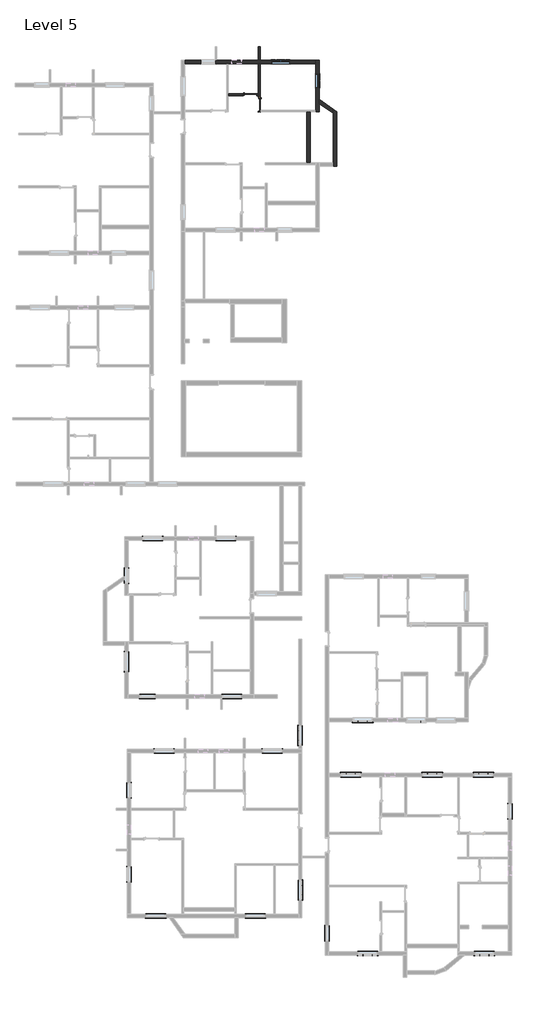
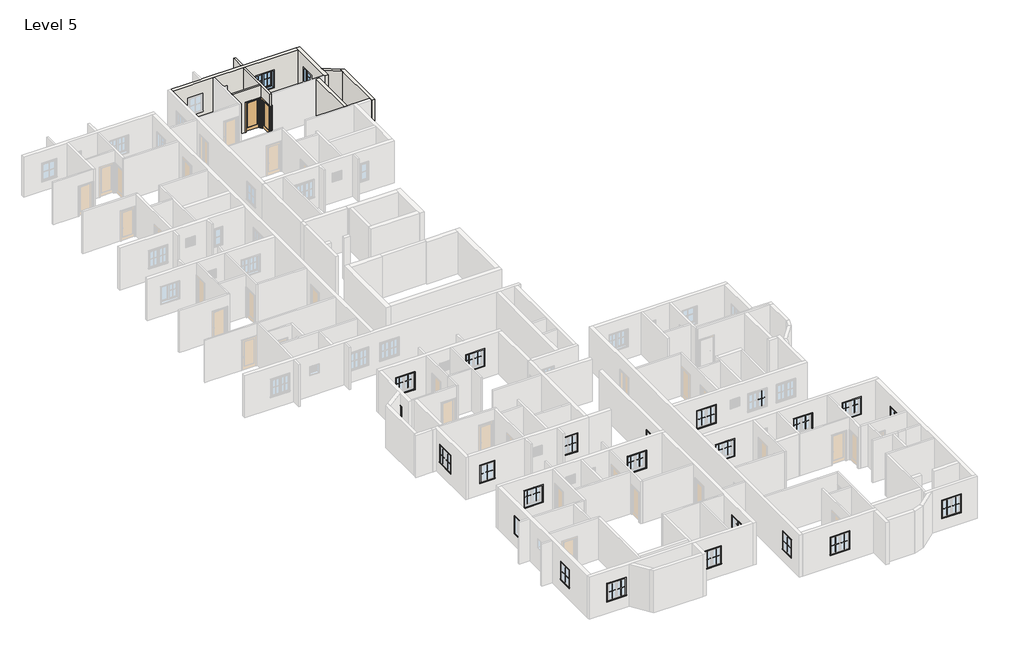
# One storey, part 6 of 7: 82 proxies, 8 walls, 2 doors, 2 windows.
"""IFC4 building model written with IfcOpenShell, lengths in millimetres."""

from ifc_helpers import new_model, si_unit, frame, origin, place, context, project, spatial, polyline, outline, extrude, faceted_brep, transform, mapped, element, save
from components import muntin_pattern_2x2_muntin_pattern_2x2_95b57395, muntin_pattern_2x2_muntin_pattern_2x2_4dfeb3f3, muntin_pattern_2x2_muntin_pattern_2x2_e852a7e4, trim_window_exterior_flat_with_sill_e4b28ec3, trim_window_exterior_flat_with_sill_7cfdd449, trim_window_interior_flat_picture_frame_39ff4276, trim_window_interior_flat_picture_frame_f1e0b15b, door_3c6ab76a, window_272f20d6, window_casement_double_4_x_4_af3140d2

model = new_model("IFC4")

# Units and contexts
model_context = context("Model", 3, world=origin())
ifc_project = project(units=[si_unit("LENGTHUNIT", "METRE", prefix="MILLI")], contexts=[model_context])

# Site, building, storey
site = spatial("IfcSite", under=ifc_project)
building = spatial("IfcBuilding", under=site)
storey = spatial("IfcBuildingStorey", under=building, Name="Level 5", Elevation=6400.8)

# Proxies
placement = place(None, origin())
muntin_pattern_2x2_muntin_pattern_2x2_shape = muntin_pattern_2x2_muntin_pattern_2x2_95b57395(model_context)
element("IfcBuildingElementProxy", 1, Name="Muntin Pattern_2x2 : Muntin Pattern_2x2", ObjectType="Muntin Pattern_2x2 : Muntin Pattern_2x2", at=placement, inside=storey, context=model_context, shape_type="MappedRepresentation", body=[
    mapped(muntin_pattern_2x2_muntin_pattern_2x2_shape, transform((17627.3240531, -20041.5997229, 7385.05), x_axis=(0.0, 1.0, 0.0), y_axis=(-1.0, 0.0, 0.0), z_axis=(0.0, 0.0, 1.0))),
])
element("IfcBuildingElementProxy", 2, Name="Muntin Pattern_2x2 : Muntin Pattern_2x2", ObjectType="Muntin Pattern_2x2 : Muntin Pattern_2x2", at=placement, inside=storey, context=model_context, shape_type="MappedRepresentation", body=[
    mapped(muntin_pattern_2x2_muntin_pattern_2x2_shape, transform((5625.8240531, -28048.9497229, 7385.05), x_axis=(0.0, 1.0, 0.0), y_axis=(-1.0, 0.0, 0.0), z_axis=(0.0, 0.0, 1.0))),
])
element("IfcBuildingElementProxy", 3, Name="Muntin Pattern_2x2 : Muntin Pattern_2x2", ObjectType="Muntin Pattern_2x2 : Muntin Pattern_2x2", at=placement, inside=storey, context=model_context, shape_type="MappedRepresentation", body=[
    mapped(muntin_pattern_2x2_muntin_pattern_2x2_shape, transform((-7378.9759469, -24172.9363256, 7385.05), x_axis=(0.0, 1.0, 0.0), y_axis=(-1.0, 0.0, 0.0), z_axis=(0.0, 0.0, 1.0))),
])
element("IfcBuildingElementProxy", 4, Name="Muntin Pattern_2x2 : Muntin Pattern_2x2", ObjectType="Muntin Pattern_2x2 : Muntin Pattern_2x2", at=placement, inside=storey, context=model_context, shape_type="MappedRepresentation", body=[
    mapped(muntin_pattern_2x2_muntin_pattern_2x2_shape, transform((-7169.4259469, -18656.0038828, 7385.05), x_axis=(0.0, -1.0, 0.0), y_axis=(1.0, 0.0, 0.0), z_axis=(0.0, 0.0, 1.0))),
])
element("IfcBuildingElementProxy", 5, Name="Muntin Pattern_2x2 : Muntin Pattern_2x2", ObjectType="Muntin Pattern_2x2 : Muntin Pattern_2x2", at=placement, inside=storey, context=model_context, shape_type="MappedRepresentation", body=[
    mapped(muntin_pattern_2x2_muntin_pattern_2x2_shape, transform((-6067.7009469, -12594.9288828, 7385.05), x_axis=(-1.0, 0.0, 0.0), y_axis=(0.0, -1.0, 0.0), z_axis=(0.0, 0.0, 1.0))),
])
element("IfcBuildingElementProxy", 6, Name="Muntin Pattern_2x2 : Muntin Pattern_2x2", ObjectType="Muntin Pattern_2x2 : Muntin Pattern_2x2", at=placement, inside=storey, context=model_context, shape_type="MappedRepresentation", body=[
    mapped(muntin_pattern_2x2_muntin_pattern_2x2_shape, transform((-7334.5259469, -4559.0038828, 7385.05), x_axis=(0.0, -1.0, 0.0), y_axis=(1.0, 0.0, 0.0), z_axis=(0.0, 0.0, 1.0))),
])
muntin_pattern_2x2_muntin_pattern_2x2_2_shape = muntin_pattern_2x2_muntin_pattern_2x2_4dfeb3f3(model_context)
element("IfcBuildingElementProxy", 7, Name="Muntin Pattern_2x2 : Muntin Pattern_2x2", ObjectType="Muntin Pattern_2x2 : Muntin Pattern_2x2", at=placement, inside=storey, context=model_context, shape_type="MappedRepresentation", body=[
    mapped(muntin_pattern_2x2_muntin_pattern_2x2_2_shape, transform((11869.4615531, -14158.3247229, 7385.05), x_axis=(-1.0, 0.0, 0.0), y_axis=(0.0, -1.0, 0.0), z_axis=(0.0, 0.0, 1.0))),
])
element("IfcBuildingElementProxy", 8, Name="Muntin Pattern_2x2 : Muntin Pattern_2x2", ObjectType="Muntin Pattern_2x2 : Muntin Pattern_2x2", at=placement, inside=storey, context=model_context, shape_type="MappedRepresentation", body=[
    mapped(muntin_pattern_2x2_muntin_pattern_2x2_2_shape, transform((8364.2615531, -14158.3247229, 7385.05), x_axis=(-1.0, 0.0, 0.0), y_axis=(0.0, -1.0, 0.0), z_axis=(0.0, 0.0, 1.0))),
])
element("IfcBuildingElementProxy", 9, Name="Muntin Pattern_2x2 : Muntin Pattern_2x2", ObjectType="Muntin Pattern_2x2 : Muntin Pattern_2x2", at=placement, inside=storey, context=model_context, shape_type="MappedRepresentation", body=[
    mapped(muntin_pattern_2x2_muntin_pattern_2x2_2_shape, transform((6976.7865531, -17530.1747229, 7385.05), x_axis=(1.0, 0.0, 0.0), y_axis=(0.0, 1.0, 0.0), z_axis=(0.0, 0.0, 1.0))),
])
element("IfcBuildingElementProxy", 10, Name="Muntin Pattern_2x2 : Muntin Pattern_2x2", ObjectType="Muntin Pattern_2x2 : Muntin Pattern_2x2", at=placement, inside=storey, context=model_context, shape_type="MappedRepresentation", body=[
    mapped(muntin_pattern_2x2_muntin_pattern_2x2_2_shape, transform((12323.4865531, -17530.1747229, 7385.05), x_axis=(1.0, 0.0, 0.0), y_axis=(0.0, 1.0, 0.0), z_axis=(0.0, 0.0, 1.0))),
])
element("IfcBuildingElementProxy", 11, Name="Muntin Pattern_2x2 : Muntin Pattern_2x2", ObjectType="Muntin Pattern_2x2 : Muntin Pattern_2x2", at=placement, inside=storey, context=model_context, shape_type="MappedRepresentation", body=[
    mapped(muntin_pattern_2x2_muntin_pattern_2x2_2_shape, transform((15682.6365531, -17530.1747229, 7385.05), x_axis=(1.0, 0.0, 0.0), y_axis=(0.0, 1.0, 0.0), z_axis=(0.0, 0.0, 1.0))),
])
element("IfcBuildingElementProxy", 12, Name="Muntin Pattern_2x2 : Muntin Pattern_2x2", ObjectType="Muntin Pattern_2x2 : Muntin Pattern_2x2", at=placement, inside=storey, context=model_context, shape_type="MappedRepresentation", body=[
    mapped(muntin_pattern_2x2_muntin_pattern_2x2_2_shape, transform((16349.3865531, -29474.5247229, 7385.05), x_axis=(-1.0, 0.0, 0.0), y_axis=(0.0, -1.0, 0.0), z_axis=(0.0, 0.0, 1.0))),
])
element("IfcBuildingElementProxy", 13, Name="Muntin Pattern_2x2 : Muntin Pattern_2x2", ObjectType="Muntin Pattern_2x2 : Muntin Pattern_2x2", at=placement, inside=storey, context=model_context, shape_type="MappedRepresentation", body=[
    mapped(muntin_pattern_2x2_muntin_pattern_2x2_2_shape, transform((8694.4615531, -29474.5247229, 7385.05), x_axis=(-1.0, 0.0, 0.0), y_axis=(0.0, -1.0, 0.0), z_axis=(0.0, 0.0, 1.0))),
])
element("IfcBuildingElementProxy", 14, Name="Muntin Pattern_2x2 : Muntin Pattern_2x2", ObjectType="Muntin Pattern_2x2 : Muntin Pattern_2x2", at=placement, inside=storey, context=model_context, shape_type="MappedRepresentation", body=[
    mapped(muntin_pattern_2x2_muntin_pattern_2x2_2_shape, transform((4070.0740531, -24902.8163828, 7385.05), x_axis=(0.0, -1.0, 0.0), y_axis=(1.0, 0.0, 0.0), z_axis=(0.0, 0.0, 1.0))),
])
element("IfcBuildingElementProxy", 15, Name="Muntin Pattern_2x2 : Muntin Pattern_2x2", ObjectType="Muntin Pattern_2x2 : Muntin Pattern_2x2", at=placement, inside=storey, context=model_context, shape_type="MappedRepresentation", body=[
    mapped(muntin_pattern_2x2_muntin_pattern_2x2_2_shape, transform((1325.2865531, -26996.7288828, 7385.05), x_axis=(-1.0, 0.0, 0.0), y_axis=(0.0, -1.0, 0.0), z_axis=(0.0, 0.0, 1.0))),
])
element("IfcBuildingElementProxy", 16, Name="Muntin Pattern_2x2 : Muntin Pattern_2x2", ObjectType="Muntin Pattern_2x2 : Muntin Pattern_2x2", at=placement, inside=storey, context=model_context, shape_type="MappedRepresentation", body=[
    mapped(muntin_pattern_2x2_muntin_pattern_2x2_2_shape, transform((-5208.8634469, -26996.7288828, 7385.05), x_axis=(-1.0, 0.0, 0.0), y_axis=(0.0, -1.0, 0.0), z_axis=(0.0, 0.0, 1.0))),
])
element("IfcBuildingElementProxy", 17, Name="Muntin Pattern_2x2 : Muntin Pattern_2x2", ObjectType="Muntin Pattern_2x2 : Muntin Pattern_2x2", at=placement, inside=storey, context=model_context, shape_type="MappedRepresentation", body=[
    mapped(muntin_pattern_2x2_muntin_pattern_2x2_2_shape, transform((1823.7615531, -15966.7788828, 7385.05), x_axis=(1.0, 0.0, 0.0), y_axis=(0.0, 1.0, 0.0), z_axis=(0.0, 0.0, 1.0))),
])
element("IfcBuildingElementProxy", 18, Name="Muntin Pattern_2x2 : Muntin Pattern_2x2", ObjectType="Muntin Pattern_2x2 : Muntin Pattern_2x2", at=placement, inside=storey, context=model_context, shape_type="MappedRepresentation", body=[
    mapped(muntin_pattern_2x2_muntin_pattern_2x2_2_shape, transform((-5272.3634469, -15966.7788828, 7385.05), x_axis=(1.0, 0.0, 0.0), y_axis=(0.0, 1.0, 0.0), z_axis=(0.0, 0.0, 1.0))),
])
element("IfcBuildingElementProxy", 19, Name="Muntin Pattern_2x2 : Muntin Pattern_2x2", ObjectType="Muntin Pattern_2x2 : Muntin Pattern_2x2", at=placement, inside=storey, context=model_context, shape_type="MappedRepresentation", body=[
    mapped(muntin_pattern_2x2_muntin_pattern_2x2_2_shape, transform((3860.5240531, -15358.7663828, 7385.05), x_axis=(0.0, 1.0, 0.0), y_axis=(-1.0, 0.0, 0.0), z_axis=(0.0, 0.0, 1.0))),
])
element("IfcBuildingElementProxy", 20, Name="Muntin Pattern_2x2 : Muntin Pattern_2x2", ObjectType="Muntin Pattern_2x2 : Muntin Pattern_2x2", at=placement, inside=storey, context=model_context, shape_type="MappedRepresentation", body=[
    mapped(muntin_pattern_2x2_muntin_pattern_2x2_2_shape, transform((-239.9884469, -12594.9288828, 7385.05), x_axis=(-1.0, 0.0, 0.0), y_axis=(0.0, -1.0, 0.0), z_axis=(0.0, 0.0, 1.0))),
])
element("IfcBuildingElementProxy", 21, Name="Muntin Pattern_2x2 : Muntin Pattern_2x2", ObjectType="Muntin Pattern_2x2 : Muntin Pattern_2x2", at=placement, inside=storey, context=model_context, shape_type="MappedRepresentation", body=[
    mapped(muntin_pattern_2x2_muntin_pattern_2x2_2_shape, transform((-7544.0759469, -10513.7163828, 7385.05), x_axis=(0.0, 1.0, 0.0), y_axis=(-1.0, 0.0, 0.0), z_axis=(0.0, 0.0, 1.0))),
])
element("IfcBuildingElementProxy", 22, Name="Muntin Pattern_2x2 : Muntin Pattern_2x2", ObjectType="Muntin Pattern_2x2 : Muntin Pattern_2x2", at=placement, inside=storey, context=model_context, shape_type="MappedRepresentation", body=[
    mapped(muntin_pattern_2x2_muntin_pattern_2x2_2_shape, transform((-6021.6634469, -2022.1788828, 7385.05), x_axis=(1.0, 0.0, 0.0), y_axis=(0.0, 1.0, 0.0), z_axis=(0.0, 0.0, 1.0))),
])
element("IfcBuildingElementProxy", 23, Name="Muntin Pattern_2x2 : Muntin Pattern_2x2", ObjectType="Muntin Pattern_2x2 : Muntin Pattern_2x2", at=placement, inside=storey, context=model_context, shape_type="MappedRepresentation", body=[
    mapped(muntin_pattern_2x2_muntin_pattern_2x2_2_shape, transform((-1221.0634469, -2022.1788828, 7385.05), x_axis=(1.0, 0.0, 0.0), y_axis=(0.0, 1.0, 0.0), z_axis=(0.0, 0.0, 1.0))),
])
muntin_pattern_2x2_muntin_pattern_2x2_3_shape = muntin_pattern_2x2_muntin_pattern_2x2_e852a7e4(model_context)
element("IfcBuildingElementProxy", 24, Name="Muntin Pattern_2x2 : Muntin Pattern_2x2", ObjectType="Muntin Pattern_2x2 : Muntin Pattern_2x2", at=placement, inside=storey, context=model_context, shape_type="MappedRepresentation", body=[
    mapped(muntin_pattern_2x2_muntin_pattern_2x2_3_shape, transform((7757.8365531, -14158.3247229, 7385.05), x_axis=(1.0, 0.0, 0.0), y_axis=(0.0, 1.0, 0.0), z_axis=(0.0, 0.0, 1.0))),
])
element("IfcBuildingElementProxy", 25, Name="Muntin Pattern_2x2 : Muntin Pattern_2x2", ObjectType="Muntin Pattern_2x2 : Muntin Pattern_2x2", at=placement, inside=storey, context=model_context, shape_type="MappedRepresentation", body=[
    mapped(muntin_pattern_2x2_muntin_pattern_2x2_3_shape, transform((7583.2115531, -17530.1747229, 7385.05), x_axis=(-1.0, 0.0, 0.0), y_axis=(0.0, -1.0, 0.0), z_axis=(0.0, 0.0, 1.0))),
])
element("IfcBuildingElementProxy", 26, Name="Muntin Pattern_2x2 : Muntin Pattern_2x2", ObjectType="Muntin Pattern_2x2 : Muntin Pattern_2x2", at=placement, inside=storey, context=model_context, shape_type="MappedRepresentation", body=[
    mapped(muntin_pattern_2x2_muntin_pattern_2x2_3_shape, transform((12929.9115531, -17530.1747229, 7385.05), x_axis=(-1.0, 0.0, 0.0), y_axis=(0.0, -1.0, 0.0), z_axis=(0.0, 0.0, 1.0))),
])
element("IfcBuildingElementProxy", 27, Name="Muntin Pattern_2x2 : Muntin Pattern_2x2", ObjectType="Muntin Pattern_2x2 : Muntin Pattern_2x2", at=placement, inside=storey, context=model_context, shape_type="MappedRepresentation", body=[
    mapped(muntin_pattern_2x2_muntin_pattern_2x2_3_shape, transform((16289.0615531, -17530.1747229, 7385.05), x_axis=(-1.0, 0.0, 0.0), y_axis=(0.0, -1.0, 0.0), z_axis=(0.0, 0.0, 1.0))),
])
element("IfcBuildingElementProxy", 28, Name="Muntin Pattern_2x2 : Muntin Pattern_2x2", ObjectType="Muntin Pattern_2x2 : Muntin Pattern_2x2", at=placement, inside=storey, context=model_context, shape_type="MappedRepresentation", body=[
    mapped(muntin_pattern_2x2_muntin_pattern_2x2_3_shape, transform((15742.9615531, -29474.5247229, 7385.05), x_axis=(1.0, 0.0, 0.0), y_axis=(0.0, 1.0, 0.0), z_axis=(0.0, 0.0, 1.0))),
])
element("IfcBuildingElementProxy", 29, Name="Muntin Pattern_2x2 : Muntin Pattern_2x2", ObjectType="Muntin Pattern_2x2 : Muntin Pattern_2x2", at=placement, inside=storey, context=model_context, shape_type="MappedRepresentation", body=[
    mapped(muntin_pattern_2x2_muntin_pattern_2x2_3_shape, transform((8088.0365531, -29474.5247229, 7385.05), x_axis=(1.0, 0.0, 0.0), y_axis=(0.0, 1.0, 0.0), z_axis=(0.0, 0.0, 1.0))),
])
element("IfcBuildingElementProxy", 30, Name="Muntin Pattern_2x2 : Muntin Pattern_2x2", ObjectType="Muntin Pattern_2x2 : Muntin Pattern_2x2", at=placement, inside=storey, context=model_context, shape_type="MappedRepresentation", body=[
    mapped(muntin_pattern_2x2_muntin_pattern_2x2_3_shape, transform((4070.0740531, -25509.2413828, 7385.05), x_axis=(0.0, 1.0, 0.0), y_axis=(-1.0, 0.0, 0.0), z_axis=(0.0, 0.0, 1.0))),
])
element("IfcBuildingElementProxy", 31, Name="Muntin Pattern_2x2 : Muntin Pattern_2x2", ObjectType="Muntin Pattern_2x2 : Muntin Pattern_2x2", at=placement, inside=storey, context=model_context, shape_type="MappedRepresentation", body=[
    mapped(muntin_pattern_2x2_muntin_pattern_2x2_3_shape, transform((718.8615531, -26996.7288828, 7385.05), x_axis=(1.0, 0.0, 0.0), y_axis=(0.0, 1.0, 0.0), z_axis=(0.0, 0.0, 1.0))),
])
element("IfcBuildingElementProxy", 32, Name="Muntin Pattern_2x2 : Muntin Pattern_2x2", ObjectType="Muntin Pattern_2x2 : Muntin Pattern_2x2", at=placement, inside=storey, context=model_context, shape_type="MappedRepresentation", body=[
    mapped(muntin_pattern_2x2_muntin_pattern_2x2_3_shape, transform((-5815.2884469, -26996.7288828, 7385.05), x_axis=(1.0, 0.0, 0.0), y_axis=(0.0, 1.0, 0.0), z_axis=(0.0, 0.0, 1.0))),
])
element("IfcBuildingElementProxy", 33, Name="Muntin Pattern_2x2 : Muntin Pattern_2x2", ObjectType="Muntin Pattern_2x2 : Muntin Pattern_2x2", at=placement, inside=storey, context=model_context, shape_type="MappedRepresentation", body=[
    mapped(muntin_pattern_2x2_muntin_pattern_2x2_3_shape, transform((2430.1865531, -15966.7788828, 7385.05), x_axis=(-1.0, 0.0, 0.0), y_axis=(0.0, -1.0, 0.0), z_axis=(0.0, 0.0, 1.0))),
])
element("IfcBuildingElementProxy", 34, Name="Muntin Pattern_2x2 : Muntin Pattern_2x2", ObjectType="Muntin Pattern_2x2 : Muntin Pattern_2x2", at=placement, inside=storey, context=model_context, shape_type="MappedRepresentation", body=[
    mapped(muntin_pattern_2x2_muntin_pattern_2x2_3_shape, transform((-4665.9384469, -15966.7788828, 7385.05), x_axis=(-1.0, 0.0, 0.0), y_axis=(0.0, -1.0, 0.0), z_axis=(0.0, 0.0, 1.0))),
])
element("IfcBuildingElementProxy", 35, Name="Muntin Pattern_2x2 : Muntin Pattern_2x2", ObjectType="Muntin Pattern_2x2 : Muntin Pattern_2x2", at=placement, inside=storey, context=model_context, shape_type="MappedRepresentation", body=[
    mapped(muntin_pattern_2x2_muntin_pattern_2x2_3_shape, transform((3860.5240531, -14752.3413828, 7385.05), x_axis=(0.0, -1.0, 0.0), y_axis=(1.0, 0.0, 0.0), z_axis=(0.0, 0.0, 1.0))),
])
element("IfcBuildingElementProxy", 36, Name="Muntin Pattern_2x2 : Muntin Pattern_2x2", ObjectType="Muntin Pattern_2x2 : Muntin Pattern_2x2", at=placement, inside=storey, context=model_context, shape_type="MappedRepresentation", body=[
    mapped(muntin_pattern_2x2_muntin_pattern_2x2_3_shape, transform((-846.4134469, -12594.9288828, 7385.05), x_axis=(1.0, 0.0, 0.0), y_axis=(0.0, 1.0, 0.0), z_axis=(0.0, 0.0, 1.0))),
])
element("IfcBuildingElementProxy", 37, Name="Muntin Pattern_2x2 : Muntin Pattern_2x2", ObjectType="Muntin Pattern_2x2 : Muntin Pattern_2x2", at=placement, inside=storey, context=model_context, shape_type="MappedRepresentation", body=[
    mapped(muntin_pattern_2x2_muntin_pattern_2x2_3_shape, transform((-7544.0759469, -9907.2913828, 7385.05), x_axis=(0.0, -1.0, 0.0), y_axis=(1.0, 0.0, 0.0), z_axis=(0.0, 0.0, 1.0))),
])
element("IfcBuildingElementProxy", 38, Name="Muntin Pattern_2x2 : Muntin Pattern_2x2", ObjectType="Muntin Pattern_2x2 : Muntin Pattern_2x2", at=placement, inside=storey, context=model_context, shape_type="MappedRepresentation", body=[
    mapped(muntin_pattern_2x2_muntin_pattern_2x2_3_shape, transform((-5415.2384469, -2022.1788828, 7385.05), x_axis=(-1.0, 0.0, 0.0), y_axis=(0.0, -1.0, 0.0), z_axis=(0.0, 0.0, 1.0))),
])
element("IfcBuildingElementProxy", 39, Name="Muntin Pattern_2x2 : Muntin Pattern_2x2", ObjectType="Muntin Pattern_2x2 : Muntin Pattern_2x2", at=placement, inside=storey, context=model_context, shape_type="MappedRepresentation", body=[
    mapped(muntin_pattern_2x2_muntin_pattern_2x2_3_shape, transform((-614.6384469, -2022.1788828, 7385.05), x_axis=(-1.0, 0.0, 0.0), y_axis=(0.0, -1.0, 0.0), z_axis=(0.0, 0.0, 1.0))),
])
trim_window_exterior_flat_with_sill_shape = trim_window_exterior_flat_with_sill_e4b28ec3(model_context)
element("IfcBuildingElementProxy", 40, Name="Trim-Window-Exterior-Flat : with Sill", ObjectType="Trim-Window-Exterior-Flat : with Sill", at=placement, inside=storey, context=model_context, shape_type="MappedRepresentation", body=[
    mapped(trim_window_exterior_flat_with_sill_shape, transform((17617.7990531, -20041.5997229, 8534.4), x_axis=(0.0, -1.0, 0.0), y_axis=(0.0, 0.0, 1.0), z_axis=(-1.0, 0.0, 0.0))),
])
element("IfcBuildingElementProxy", 41, Name="Trim-Window-Exterior-Flat : with Sill", ObjectType="Trim-Window-Exterior-Flat : with Sill", at=placement, inside=storey, context=model_context, shape_type="MappedRepresentation", body=[
    mapped(trim_window_exterior_flat_with_sill_shape, transform((5616.2990531, -28048.9497229, 8534.4), x_axis=(0.0, -1.0, 0.0), y_axis=(0.0, 0.0, 1.0), z_axis=(-1.0, 0.0, 0.0))),
])
element("IfcBuildingElementProxy", 42, Name="Trim-Window-Exterior-Flat : with Sill", ObjectType="Trim-Window-Exterior-Flat : with Sill", at=placement, inside=storey, context=model_context, shape_type="MappedRepresentation", body=[
    mapped(trim_window_exterior_flat_with_sill_shape, transform((-7388.5009469, -24172.9363256, 8534.4), x_axis=(0.0, -1.0, 0.0), y_axis=(0.0, 0.0, 1.0), z_axis=(-1.0, 0.0, 0.0))),
])
element("IfcBuildingElementProxy", 43, Name="Trim-Window-Exterior-Flat : with Sill", ObjectType="Trim-Window-Exterior-Flat : with Sill", at=placement, inside=storey, context=model_context, shape_type="MappedRepresentation", body=[
    mapped(trim_window_exterior_flat_with_sill_shape, transform((-7159.9009469, -18656.0038828, 8534.4), x_axis=(0.0, 1.0, 0.0), y_axis=(0.0, 0.0, 1.0), z_axis=(1.0, 0.0, 0.0))),
])
element("IfcBuildingElementProxy", 44, Name="Trim-Window-Exterior-Flat : with Sill", ObjectType="Trim-Window-Exterior-Flat : with Sill", at=placement, inside=storey, context=model_context, shape_type="MappedRepresentation", body=[
    mapped(trim_window_exterior_flat_with_sill_shape, transform((-6067.7009469, -12604.4538828, 8534.4), x_axis=(1.0, 0.0, 0.0), y_axis=(0.0, 0.0, 1.0), z_axis=(0.0, -1.0, 0.0))),
])
element("IfcBuildingElementProxy", 45, Name="Trim-Window-Exterior-Flat : with Sill", ObjectType="Trim-Window-Exterior-Flat : with Sill", at=placement, inside=storey, context=model_context, shape_type="MappedRepresentation", body=[
    mapped(trim_window_exterior_flat_with_sill_shape, transform((-7325.0009469, -4559.0038828, 8534.4), x_axis=(0.0, 1.0, 0.0), y_axis=(0.0, 0.0, 1.0), z_axis=(1.0, 0.0, 0.0))),
])
trim_window_exterior_flat_with_sill_2_shape = trim_window_exterior_flat_with_sill_7cfdd449(model_context)
element("IfcBuildingElementProxy", 46, Name="Trim-Window-Exterior-Flat : with Sill", ObjectType="Trim-Window-Exterior-Flat : with Sill", at=placement, inside=storey, context=model_context, shape_type="MappedRepresentation", body=[
    mapped(trim_window_exterior_flat_with_sill_2_shape, transform((8061.0490531, -14167.8497229, 8534.4), x_axis=(1.0, 0.0, 0.0), y_axis=(0.0, 0.0, 1.0), z_axis=(0.0, -1.0, 0.0))),
])
element("IfcBuildingElementProxy", 47, Name="Trim-Window-Exterior-Flat : with Sill", ObjectType="Trim-Window-Exterior-Flat : with Sill", at=placement, inside=storey, context=model_context, shape_type="MappedRepresentation", body=[
    mapped(trim_window_exterior_flat_with_sill_2_shape, transform((7279.9990531, -17520.6497229, 8534.4), x_axis=(-1.0, 0.0, 0.0), y_axis=(0.0, 0.0, 1.0), z_axis=(0.0, 1.0, 0.0))),
])
element("IfcBuildingElementProxy", 48, Name="Trim-Window-Exterior-Flat : with Sill", ObjectType="Trim-Window-Exterior-Flat : with Sill", at=placement, inside=storey, context=model_context, shape_type="MappedRepresentation", body=[
    mapped(trim_window_exterior_flat_with_sill_2_shape, transform((12626.6990531, -17520.6497229, 8534.4), x_axis=(-1.0, 0.0, 0.0), y_axis=(0.0, 0.0, 1.0), z_axis=(0.0, 1.0, 0.0))),
])
element("IfcBuildingElementProxy", 49, Name="Trim-Window-Exterior-Flat : with Sill", ObjectType="Trim-Window-Exterior-Flat : with Sill", at=placement, inside=storey, context=model_context, shape_type="MappedRepresentation", body=[
    mapped(trim_window_exterior_flat_with_sill_2_shape, transform((15985.8490531, -17520.6497229, 8534.4), x_axis=(-1.0, 0.0, 0.0), y_axis=(0.0, 0.0, 1.0), z_axis=(0.0, 1.0, 0.0))),
])
element("IfcBuildingElementProxy", 50, Name="Trim-Window-Exterior-Flat : with Sill", ObjectType="Trim-Window-Exterior-Flat : with Sill", at=placement, inside=storey, context=model_context, shape_type="MappedRepresentation", body=[
    mapped(trim_window_exterior_flat_with_sill_2_shape, transform((16046.1740531, -29484.0497229, 8534.4), x_axis=(1.0, 0.0, 0.0), y_axis=(0.0, 0.0, 1.0), z_axis=(0.0, -1.0, 0.0))),
])
element("IfcBuildingElementProxy", 51, Name="Trim-Window-Exterior-Flat : with Sill", ObjectType="Trim-Window-Exterior-Flat : with Sill", at=placement, inside=storey, context=model_context, shape_type="MappedRepresentation", body=[
    mapped(trim_window_exterior_flat_with_sill_2_shape, transform((8391.2490531, -29484.0497229, 8534.4), x_axis=(1.0, 0.0, 0.0), y_axis=(0.0, 0.0, 1.0), z_axis=(0.0, -1.0, 0.0))),
])
element("IfcBuildingElementProxy", 52, Name="Trim-Window-Exterior-Flat : with Sill", ObjectType="Trim-Window-Exterior-Flat : with Sill", at=placement, inside=storey, context=model_context, shape_type="MappedRepresentation", body=[
    mapped(trim_window_exterior_flat_with_sill_2_shape, transform((4079.5990531, -25206.0288828, 8534.4), x_axis=(0.0, 1.0, 0.0), y_axis=(0.0, 0.0, 1.0), z_axis=(1.0, 0.0, 0.0))),
])
element("IfcBuildingElementProxy", 53, Name="Trim-Window-Exterior-Flat : with Sill", ObjectType="Trim-Window-Exterior-Flat : with Sill", at=placement, inside=storey, context=model_context, shape_type="MappedRepresentation", body=[
    mapped(trim_window_exterior_flat_with_sill_2_shape, transform((1022.0740531, -27006.2538828, 8534.4), x_axis=(1.0, 0.0, 0.0), y_axis=(0.0, 0.0, 1.0), z_axis=(0.0, -1.0, 0.0))),
])
element("IfcBuildingElementProxy", 54, Name="Trim-Window-Exterior-Flat : with Sill", ObjectType="Trim-Window-Exterior-Flat : with Sill", at=placement, inside=storey, context=model_context, shape_type="MappedRepresentation", body=[
    mapped(trim_window_exterior_flat_with_sill_2_shape, transform((-5512.0759469, -27006.2538828, 8534.4), x_axis=(1.0, 0.0, 0.0), y_axis=(0.0, 0.0, 1.0), z_axis=(0.0, -1.0, 0.0))),
])
element("IfcBuildingElementProxy", 55, Name="Trim-Window-Exterior-Flat : with Sill", ObjectType="Trim-Window-Exterior-Flat : with Sill", at=placement, inside=storey, context=model_context, shape_type="MappedRepresentation", body=[
    mapped(trim_window_exterior_flat_with_sill_2_shape, transform((2126.9740531, -15957.2538828, 8534.4), x_axis=(-1.0, 0.0, 0.0), y_axis=(0.0, 0.0, 1.0), z_axis=(0.0, 1.0, 0.0))),
])
element("IfcBuildingElementProxy", 56, Name="Trim-Window-Exterior-Flat : with Sill", ObjectType="Trim-Window-Exterior-Flat : with Sill", at=placement, inside=storey, context=model_context, shape_type="MappedRepresentation", body=[
    mapped(trim_window_exterior_flat_with_sill_2_shape, transform((-4969.1509469, -15957.2538828, 8534.4), x_axis=(-1.0, 0.0, 0.0), y_axis=(0.0, 0.0, 1.0), z_axis=(0.0, 1.0, 0.0))),
])
element("IfcBuildingElementProxy", 57, Name="Trim-Window-Exterior-Flat : with Sill", ObjectType="Trim-Window-Exterior-Flat : with Sill", at=placement, inside=storey, context=model_context, shape_type="MappedRepresentation", body=[
    mapped(trim_window_exterior_flat_with_sill_2_shape, transform((3850.9990531, -15055.5538828, 8534.4), x_axis=(0.0, -1.0, 0.0), y_axis=(0.0, 0.0, 1.0), z_axis=(-1.0, 0.0, 0.0))),
])
element("IfcBuildingElementProxy", 58, Name="Trim-Window-Exterior-Flat : with Sill", ObjectType="Trim-Window-Exterior-Flat : with Sill", at=placement, inside=storey, context=model_context, shape_type="MappedRepresentation", body=[
    mapped(trim_window_exterior_flat_with_sill_2_shape, transform((-543.2009469, -12604.4538828, 8534.4), x_axis=(1.0, 0.0, 0.0), y_axis=(0.0, 0.0, 1.0), z_axis=(0.0, -1.0, 0.0))),
])
element("IfcBuildingElementProxy", 59, Name="Trim-Window-Exterior-Flat : with Sill", ObjectType="Trim-Window-Exterior-Flat : with Sill", at=placement, inside=storey, context=model_context, shape_type="MappedRepresentation", body=[
    mapped(trim_window_exterior_flat_with_sill_2_shape, transform((-7553.6009469, -10210.5038828, 8534.4), x_axis=(0.0, -1.0, 0.0), y_axis=(0.0, 0.0, 1.0), z_axis=(-1.0, 0.0, 0.0))),
])
element("IfcBuildingElementProxy", 60, Name="Trim-Window-Exterior-Flat : with Sill", ObjectType="Trim-Window-Exterior-Flat : with Sill", at=placement, inside=storey, context=model_context, shape_type="MappedRepresentation", body=[
    mapped(trim_window_exterior_flat_with_sill_2_shape, transform((-5718.4509469, -2012.6538828, 8534.4), x_axis=(-1.0, 0.0, 0.0), y_axis=(0.0, 0.0, 1.0), z_axis=(0.0, 1.0, 0.0))),
])
element("IfcBuildingElementProxy", 61, Name="Trim-Window-Exterior-Flat : with Sill", ObjectType="Trim-Window-Exterior-Flat : with Sill", at=placement, inside=storey, context=model_context, shape_type="MappedRepresentation", body=[
    mapped(trim_window_exterior_flat_with_sill_2_shape, transform((-917.8509469, -2012.6538828, 8534.4), x_axis=(-1.0, 0.0, 0.0), y_axis=(0.0, 0.0, 1.0), z_axis=(0.0, 1.0, 0.0))),
])
trim_window_interior_flat_picture_frame_shape = trim_window_interior_flat_picture_frame_39ff4276(model_context)
element("IfcBuildingElementProxy", 62, Name="Trim-Window-Interior-Flat : Picture Frame", ObjectType="Trim-Window-Interior-Flat : Picture Frame", at=placement, inside=storey, context=model_context, shape_type="MappedRepresentation", body=[
    mapped(trim_window_interior_flat_picture_frame_shape, transform((17846.3990531, -20041.5997229, 8534.4), x_axis=(0.0, 1.0, 0.0), y_axis=(0.0, 0.0, 1.0), z_axis=(1.0, 0.0, 0.0))),
])
element("IfcBuildingElementProxy", 63, Name="Trim-Window-Interior-Flat : Picture Frame", ObjectType="Trim-Window-Interior-Flat : Picture Frame", at=placement, inside=storey, context=model_context, shape_type="MappedRepresentation", body=[
    mapped(trim_window_interior_flat_picture_frame_shape, transform((5844.8990531, -28048.9497229, 8534.4), x_axis=(0.0, 1.0, 0.0), y_axis=(0.0, 0.0, 1.0), z_axis=(1.0, 0.0, 0.0))),
])
element("IfcBuildingElementProxy", 64, Name="Trim-Window-Interior-Flat : Picture Frame", ObjectType="Trim-Window-Interior-Flat : Picture Frame", at=placement, inside=storey, context=model_context, shape_type="MappedRepresentation", body=[
    mapped(trim_window_interior_flat_picture_frame_shape, transform((-7159.9009469, -24172.9363256, 8534.4), x_axis=(0.0, 1.0, 0.0), y_axis=(0.0, 0.0, 1.0), z_axis=(1.0, 0.0, 0.0))),
])
element("IfcBuildingElementProxy", 65, Name="Trim-Window-Interior-Flat : Picture Frame", ObjectType="Trim-Window-Interior-Flat : Picture Frame", at=placement, inside=storey, context=model_context, shape_type="MappedRepresentation", body=[
    mapped(trim_window_interior_flat_picture_frame_shape, transform((-7388.5009469, -18656.0038828, 8534.4), x_axis=(0.0, -1.0, 0.0), y_axis=(0.0, 0.0, 1.0), z_axis=(-1.0, 0.0, 0.0))),
])
element("IfcBuildingElementProxy", 66, Name="Trim-Window-Interior-Flat : Picture Frame", ObjectType="Trim-Window-Interior-Flat : Picture Frame", at=placement, inside=storey, context=model_context, shape_type="MappedRepresentation", body=[
    mapped(trim_window_interior_flat_picture_frame_shape, transform((-6067.7009469, -12375.8538828, 8534.4), x_axis=(-1.0, 0.0, 0.0), y_axis=(0.0, 0.0, 1.0), z_axis=(0.0, 1.0, 0.0))),
])
element("IfcBuildingElementProxy", 67, Name="Trim-Window-Interior-Flat : Picture Frame", ObjectType="Trim-Window-Interior-Flat : Picture Frame", at=placement, inside=storey, context=model_context, shape_type="MappedRepresentation", body=[
    mapped(trim_window_interior_flat_picture_frame_shape, transform((-7553.6009469, -4559.0038828, 8534.4), x_axis=(0.0, -1.0, 0.0), y_axis=(0.0, 0.0, 1.0), z_axis=(-1.0, 0.0, 0.0))),
])
trim_window_interior_flat_picture_frame_2_shape = trim_window_interior_flat_picture_frame_f1e0b15b(model_context)
element("IfcBuildingElementProxy", 68, Name="Trim-Window-Interior-Flat : Picture Frame", ObjectType="Trim-Window-Interior-Flat : Picture Frame", at=placement, inside=storey, context=model_context, shape_type="MappedRepresentation", body=[
    mapped(trim_window_interior_flat_picture_frame_2_shape, transform((7279.9990531, -17749.2497229, 8534.4), x_axis=(1.0, 0.0, 0.0), y_axis=(0.0, 0.0, 1.0), z_axis=(0.0, -1.0, 0.0))),
])
element("IfcBuildingElementProxy", 69, Name="Trim-Window-Interior-Flat : Picture Frame", ObjectType="Trim-Window-Interior-Flat : Picture Frame", at=placement, inside=storey, context=model_context, shape_type="MappedRepresentation", body=[
    mapped(trim_window_interior_flat_picture_frame_2_shape, transform((12626.6990531, -17749.2497229, 8534.4), x_axis=(1.0, 0.0, 0.0), y_axis=(0.0, 0.0, 1.0), z_axis=(0.0, -1.0, 0.0))),
])
element("IfcBuildingElementProxy", 70, Name="Trim-Window-Interior-Flat : Picture Frame", ObjectType="Trim-Window-Interior-Flat : Picture Frame", at=placement, inside=storey, context=model_context, shape_type="MappedRepresentation", body=[
    mapped(trim_window_interior_flat_picture_frame_2_shape, transform((15985.8490531, -17749.2497229, 8534.4), x_axis=(1.0, 0.0, 0.0), y_axis=(0.0, 0.0, 1.0), z_axis=(0.0, -1.0, 0.0))),
])
element("IfcBuildingElementProxy", 71, Name="Trim-Window-Interior-Flat : Picture Frame", ObjectType="Trim-Window-Interior-Flat : Picture Frame", at=placement, inside=storey, context=model_context, shape_type="MappedRepresentation", body=[
    mapped(trim_window_interior_flat_picture_frame_2_shape, transform((16046.1740531, -29255.4497229, 8534.4), x_axis=(-1.0, 0.0, 0.0), y_axis=(0.0, 0.0, 1.0), z_axis=(0.0, 1.0, 0.0))),
])
element("IfcBuildingElementProxy", 72, Name="Trim-Window-Interior-Flat : Picture Frame", ObjectType="Trim-Window-Interior-Flat : Picture Frame", at=placement, inside=storey, context=model_context, shape_type="MappedRepresentation", body=[
    mapped(trim_window_interior_flat_picture_frame_2_shape, transform((8391.2490531, -29255.4497229, 8534.4), x_axis=(-1.0, 0.0, 0.0), y_axis=(0.0, 0.0, 1.0), z_axis=(0.0, 1.0, 0.0))),
])
element("IfcBuildingElementProxy", 73, Name="Trim-Window-Interior-Flat : Picture Frame", ObjectType="Trim-Window-Interior-Flat : Picture Frame", at=placement, inside=storey, context=model_context, shape_type="MappedRepresentation", body=[
    mapped(trim_window_interior_flat_picture_frame_2_shape, transform((3850.9990531, -25206.0288828, 8534.4), x_axis=(0.0, -1.0, 0.0), y_axis=(0.0, 0.0, 1.0), z_axis=(-1.0, 0.0, 0.0))),
])
element("IfcBuildingElementProxy", 74, Name="Trim-Window-Interior-Flat : Picture Frame", ObjectType="Trim-Window-Interior-Flat : Picture Frame", at=placement, inside=storey, context=model_context, shape_type="MappedRepresentation", body=[
    mapped(trim_window_interior_flat_picture_frame_2_shape, transform((1022.0740531, -26777.6538828, 8534.4), x_axis=(-1.0, 0.0, 0.0), y_axis=(0.0, 0.0, 1.0), z_axis=(0.0, 1.0, 0.0))),
])
element("IfcBuildingElementProxy", 75, Name="Trim-Window-Interior-Flat : Picture Frame", ObjectType="Trim-Window-Interior-Flat : Picture Frame", at=placement, inside=storey, context=model_context, shape_type="MappedRepresentation", body=[
    mapped(trim_window_interior_flat_picture_frame_2_shape, transform((-5512.0759469, -26777.6538828, 8534.4), x_axis=(-1.0, 0.0, 0.0), y_axis=(0.0, 0.0, 1.0), z_axis=(0.0, 1.0, 0.0))),
])
element("IfcBuildingElementProxy", 76, Name="Trim-Window-Interior-Flat : Picture Frame", ObjectType="Trim-Window-Interior-Flat : Picture Frame", at=placement, inside=storey, context=model_context, shape_type="MappedRepresentation", body=[
    mapped(trim_window_interior_flat_picture_frame_2_shape, transform((2126.9740531, -16185.8538828, 8534.4), x_axis=(1.0, 0.0, 0.0), y_axis=(0.0, 0.0, 1.0), z_axis=(0.0, -1.0, 0.0))),
])
element("IfcBuildingElementProxy", 77, Name="Trim-Window-Interior-Flat : Picture Frame", ObjectType="Trim-Window-Interior-Flat : Picture Frame", at=placement, inside=storey, context=model_context, shape_type="MappedRepresentation", body=[
    mapped(trim_window_interior_flat_picture_frame_2_shape, transform((-4969.1509469, -16185.8538828, 8534.4), x_axis=(1.0, 0.0, 0.0), y_axis=(0.0, 0.0, 1.0), z_axis=(0.0, -1.0, 0.0))),
])
element("IfcBuildingElementProxy", 78, Name="Trim-Window-Interior-Flat : Picture Frame", ObjectType="Trim-Window-Interior-Flat : Picture Frame", at=placement, inside=storey, context=model_context, shape_type="MappedRepresentation", body=[
    mapped(trim_window_interior_flat_picture_frame_2_shape, transform((4079.5990531, -15055.5538828, 8534.4), x_axis=(0.0, 1.0, 0.0), y_axis=(0.0, 0.0, 1.0), z_axis=(1.0, 0.0, 0.0))),
])
element("IfcBuildingElementProxy", 79, Name="Trim-Window-Interior-Flat : Picture Frame", ObjectType="Trim-Window-Interior-Flat : Picture Frame", at=placement, inside=storey, context=model_context, shape_type="MappedRepresentation", body=[
    mapped(trim_window_interior_flat_picture_frame_2_shape, transform((-543.2009469, -12375.8538828, 8534.4), x_axis=(-1.0, 0.0, 0.0), y_axis=(0.0, 0.0, 1.0), z_axis=(0.0, 1.0, 0.0))),
])
element("IfcBuildingElementProxy", 80, Name="Trim-Window-Interior-Flat : Picture Frame", ObjectType="Trim-Window-Interior-Flat : Picture Frame", at=placement, inside=storey, context=model_context, shape_type="MappedRepresentation", body=[
    mapped(trim_window_interior_flat_picture_frame_2_shape, transform((-7325.0009469, -10210.5038828, 8534.4), x_axis=(0.0, 1.0, 0.0), y_axis=(0.0, 0.0, 1.0), z_axis=(1.0, 0.0, 0.0))),
])
element("IfcBuildingElementProxy", 81, Name="Trim-Window-Interior-Flat : Picture Frame", ObjectType="Trim-Window-Interior-Flat : Picture Frame", at=placement, inside=storey, context=model_context, shape_type="MappedRepresentation", body=[
    mapped(trim_window_interior_flat_picture_frame_2_shape, transform((-5718.4509469, -2241.2538828, 8534.4), x_axis=(1.0, 0.0, 0.0), y_axis=(0.0, 0.0, 1.0), z_axis=(0.0, -1.0, 0.0))),
])
element("IfcBuildingElementProxy", 82, Name="Trim-Window-Interior-Flat : Picture Frame", ObjectType="Trim-Window-Interior-Flat : Picture Frame", at=placement, inside=storey, context=model_context, shape_type="MappedRepresentation", body=[
    mapped(trim_window_interior_flat_picture_frame_2_shape, transform((-917.8509469, -2241.2538828, 8534.4), x_axis=(1.0, 0.0, 0.0), y_axis=(0.0, 0.0, 1.0), z_axis=(0.0, -1.0, 0.0))),
])

# Doors
door_shape = door_3c6ab76a(model_context)
element("IfcDoor", 83, ObjectType="Door-Interior-Single-1_Panel-Wood : 2'6\" x 7' door", at=placement, inside=storey, context=model_context, shape_type="MappedRepresentation", body=[
    mapped(door_shape, transform((669.6490531, 27005.8505084, 6400.8), x_axis=(1.0, 0.0, 0.0), y_axis=(0.0, 1.0, 0.0), z_axis=(0.0, 0.0, 1.0))),
])
element("IfcDoor", 84, ObjectType="Door-Interior-Single-1_Panel-Wood : 36\" x 84\"", at=placement, inside=storey, context=model_context, shape_type="MappedRepresentation", body=[
    mapped(door_shape, transform((1282.4240531, 26367.6755084, 6400.8), x_axis=(0.0, -1.0, 0.0), y_axis=(1.0, 0.0, 0.0), z_axis=(0.0, 0.0, 1.0))),
])

# Walls
element("IfcWall", 85, ObjectType="4.5\" wall", at=placement, inside=storey, context=model_context, shape_type="Brep", body=[
    faceted_brep([(1336.3990531, 29041.0255084, 9448.8), (1336.3990531, 25993.0255084, 9448.8), (1336.3990531, 25878.7255084, 9448.8), (1336.3990531, 25878.7255084, 6400.8), (1336.3990531, 25885.0755084, 6400.8), (1336.3990531, 25885.0755084, 8559.8), (1336.3990531, 26850.2755084, 8559.8), (1336.3990531, 26850.2755084, 6400.8), (1336.3990531, 29041.0255084, 6400.8), (1222.0990531, 25878.7255084, 9448.8), (1222.0990531, 26945.5255084, 9448.8), (1222.0990531, 27059.8255084, 9448.8), (1222.0990531, 29041.0255084, 9448.8), (1222.0990531, 29041.0255084, 6400.8), (1222.0990531, 27059.8255084, 6400.8), (1222.0990531, 26945.5255084, 6400.8), (1222.0990531, 26850.2755084, 6400.8), (1222.0990531, 26850.2755084, 8559.8), (1222.0990531, 25885.0755084, 8559.8), (1222.0990531, 25885.0755084, 6400.8), (1222.0990531, 25878.7255084, 6400.8)], [[[0, 1, 2, 3, 4, 5, 6, 7, 8]], [[9, 10, 11, 12, 13, 14, 15, 16, 17, 18, 19, 20]], [[13, 8, 7, 16, 15, 14]], [[3, 20, 19, 4]], [[2, 1, 0, 12, 11, 10, 9]], [[0, 8, 13, 12]], [[3, 2, 9, 20]], [[18, 5, 4, 19]], [[5, 18, 17, 6]], [[6, 17, 16, 7]]]),
])
element("IfcWall", 86, ObjectType="4.5\" wall", at=placement, inside=storey, context=model_context, shape_type="SweptSolid", body=[
    extrude(outline(polyline([(9448.8, 1222.0990531), (9448.8, -759.1009469), (6400.8, -759.1009469), (6400.8, 187.0490531), (8559.8, 187.0490531), (8559.8, 1152.2490531), (6400.8, 1152.2490531), (6400.8, 1222.0990531), (9448.8, 1222.0990531)])), frame((0.0, 26945.5255084, 0.0), z_axis=(0.0, 1.0, 0.0), x_axis=(0.0, 0.0, 1.0)), (0.0, 0.0, 1.0), 114.3),
])
element("IfcWall", 87, ObjectType="4.5\" wall", at=placement, inside=storey, context=model_context, shape_type="SweptSolid", body=[
    extrude(outline(polyline([(1336.3990531, 30161.6889788), (1336.3990531, 29269.6255084), (1222.0990531, 29269.6255084), (1222.0990531, 30161.6889788), (1336.3990531, 30161.6889788)])), frame((0.0, 0.0, 6400.8), z_axis=(0.0, 0.0, 1.0), x_axis=(1.0, 0.0, 0.0)), (0.0, 0.0, 1.0), 3048.0),
])
element("IfcWall", 88, ObjectType="9\"", at=placement, inside=storey, context=model_context, shape_type="Brep", body=[
    faceted_brep([(-3616.6009469, 29041.0255084, 6400.8), (-873.4009469, 29041.0255084, 6400.8), (-759.1009469, 29041.0255084, 6400.8), (1222.0990531, 29041.0255084, 6400.8), (1336.3990531, 29041.0255084, 6400.8), (4993.9990531, 29041.0255084, 6400.8), (4993.9990531, 29041.0255084, 9448.8), (1336.3990531, 29041.0255084, 9448.8), (1222.0990531, 29041.0255084, 9448.8), (-759.1009469, 29041.0255084, 9448.8), (-873.4009469, 29041.0255084, 9448.8), (-3616.6009469, 29041.0255084, 9448.8), (91.7990531, 29041.0255084, 8534.4), (91.7990531, 29041.0255084, 7924.8), (-517.8009469, 29041.0255084, 7924.8), (-517.8009469, 29041.0255084, 8534.4), (-2532.2862554, 29041.0255084, 8534.4), (-1617.8862554, 29041.0255084, 8534.4), (-1617.8862554, 29041.0255084, 7315.2), (-2532.2862554, 29041.0255084, 7315.2), (3285.8490531, 29041.0255084, 8534.4), (3285.8490531, 29041.0255084, 7315.2), (2066.6490531, 29041.0255084, 7315.2), (2066.6490531, 29041.0255084, 8534.4), (-3616.6009469, 29269.6255084, 6400.8), (-3616.6009469, 29269.6255084, 9448.8), (-1617.8862554, 29269.6255084, 9448.8), (-1503.5862554, 29269.6255084, 9448.8), (1222.0990531, 29269.6255084, 9448.8), (1336.3990531, 29269.6255084, 9448.8), (4993.9990531, 29269.6255084, 9448.8), (4993.9990531, 29269.6255084, 6400.8), (1336.3990531, 29269.6255084, 6400.8), (1222.0990531, 29269.6255084, 6400.8), (-1503.5862554, 29269.6255084, 6400.8), (-1617.8862554, 29269.6255084, 6400.8), (91.7990531, 29269.6255084, 8534.4), (-517.8009469, 29269.6255084, 8534.4), (-517.8009469, 29269.6255084, 7924.8), (91.7990531, 29269.6255084, 7924.8), (-2532.2862554, 29269.6255084, 8534.4), (-2532.2862554, 29269.6255084, 7315.2), (-1617.8862554, 29269.6255084, 7315.2), (-1617.8862554, 29269.6255084, 8534.4), (3285.8490531, 29269.6255084, 8534.4), (2066.6490531, 29269.6255084, 8534.4), (2066.6490531, 29269.6255084, 7315.2), (3285.8490531, 29269.6255084, 7315.2)], [[[0, 1, 2, 3, 4, 5, 6, 7, 8, 9, 10, 11], [12, 13, 14, 15], [16, 17, 18, 19], [20, 21, 22, 23]], [[24, 25, 26, 27, 28, 29, 30, 31, 32, 33, 34, 35], [36, 37, 38, 39], [40, 41, 42, 43], [44, 45, 46, 47]], [[5, 4, 3, 2, 1, 0, 24, 35, 34, 33, 32, 31]], [[11, 10, 9, 8, 7, 6, 30, 29, 28, 27, 26, 25]], [[0, 11, 25, 24]], [[6, 5, 31, 30]], [[13, 12, 36, 39]], [[14, 13, 39, 38]], [[15, 14, 38, 37]], [[12, 15, 37, 36]], [[41, 40, 16, 19]], [[42, 41, 19, 18]], [[43, 42, 18, 17]], [[40, 43, 17, 16]], [[21, 20, 44, 47]], [[22, 21, 47, 46]], [[23, 22, 46, 45]], [[20, 23, 45, 44]]]),
])
element("IfcWall", 89, ObjectType="9\"", at=placement, inside=storey, context=model_context, shape_type="Brep", body=[
    faceted_brep([(5222.5990531, 25878.7255084, 6400.8), (5222.5990531, 26412.1255084, 6400.8), (5222.5990531, 26691.1673698, 6400.8), (5222.5990531, 29269.6255084, 6400.8), (5222.5990531, 29269.6255084, 9448.8), (5222.5990531, 26691.1673698, 9448.8), (5222.5990531, 26412.1255084, 9448.8), (5222.5990531, 25878.7255084, 9448.8), (5222.5990531, 27453.5255084, 8534.4), (5222.5990531, 28367.9255084, 8534.4), (5222.5990531, 28367.9255084, 7315.2), (5222.5990531, 27453.5255084, 7315.2), (4993.9990531, 25878.7255084, 6400.8), (4993.9990531, 25878.7255084, 9448.8), (4993.9990531, 25993.0255084, 9448.8), (4993.9990531, 29041.0255084, 9448.8), (4993.9990531, 29269.6255084, 9448.8), (4993.9990531, 29269.6255084, 6400.8), (4993.9990531, 29041.0255084, 6400.8), (4993.9990531, 25993.0255084, 6400.8), (4993.9990531, 27453.5255084, 8534.4), (4993.9990531, 27453.5255084, 7315.2), (4993.9990531, 28367.9255084, 7315.2), (4993.9990531, 28367.9255084, 8534.4)], [[[0, 1, 2, 3, 4, 5, 6, 7], [8, 9, 10, 11]], [[12, 13, 14, 15, 16, 17, 18, 19], [20, 21, 22, 23]], [[3, 2, 1, 0, 12, 19, 18, 17]], [[7, 6, 5, 4, 16, 15, 14, 13]], [[4, 3, 17, 16]], [[0, 7, 13, 12]], [[21, 20, 8, 11]], [[22, 21, 11, 10]], [[23, 22, 10, 9]], [[20, 23, 9, 8]]]),
])
element("IfcWall", 90, ObjectType="9\"", at=placement, inside=storey, context=model_context, shape_type="SweptSolid", body=[
    extrude(outline(polyline([(4612.9990531, 25878.7255084), (4612.9990531, 22525.9255084), (4384.3990531, 22525.9255084), (4384.3990531, 25878.7255084), (4612.9990531, 25878.7255084)])), frame((0.0, 0.0, 6400.8), z_axis=(0.0, 0.0, 1.0), x_axis=(1.0, 0.0, 0.0)), (0.0, 0.0, 1.0), 3048.0),
])
element("IfcWall", 91, ObjectType="9\"", at=placement, inside=storey, context=model_context, shape_type="Brep", body=[
    faceted_brep([(6136.9990531, 26051.0873698, 6400.8), (6136.9990531, 25772.0455084, 6400.8), (6136.9990531, 22525.9255084, 6400.8), (6136.9990531, 22297.3255084, 6400.8), (6136.9990531, 22297.3255084, 9448.8), (6136.9990531, 22525.9255084, 9448.8), (6136.9990531, 25772.0455084, 9448.8), (6136.9990531, 26051.0873698, 9448.8), (6365.5990531, 25891.0673698, 6400.8), (6365.5990531, 25891.0673698, 9448.8), (6365.5990531, 22297.3255084, 9448.8), (6365.5990531, 22297.3255084, 6400.8)], [[[0, 1, 2, 3, 4, 5, 6, 7]], [[8, 9, 10, 11]], [[3, 2, 1, 0, 8, 11]], [[7, 6, 5, 4, 10, 9]], [[4, 3, 11, 10]], [[0, 7, 9, 8]]]),
])
element("IfcWall", 92, ObjectType="9\"", at=placement, inside=storey, context=model_context, shape_type="SweptSolid", body=[
    extrude(outline(polyline([(6136.9990531, 25772.0455084), (5222.5990531, 26412.1255084), (5222.5990531, 26691.1673698), (6136.9990531, 26051.0873698), (6136.9990531, 25772.0455084)])), frame((0.0, 0.0, 6400.8), z_axis=(0.0, 0.0, 1.0), x_axis=(1.0, 0.0, 0.0)), (0.0, 0.0, 1.0), 3048.0),
])

# Windows
window_shape = window_272f20d6(model_context)
element("IfcWindow", 93, ObjectType="Window-Awning-Single : 36\" x 48\"", at=placement, inside=storey, context=model_context, shape_type="MappedRepresentation", body=[
    mapped(window_shape, transform((5108.2990531, 27910.7255084, 6400.8), x_axis=(0.0, -1.0, 0.0), y_axis=(1.0, 0.0, 0.0), z_axis=(0.0, 0.0, 1.0))),
])
window_casement_double_4_x_4_shape = window_casement_double_4_x_4_af3140d2(model_context)
element("IfcWindow", 94, ObjectType="Window-Casement-Double : 4' x 4'", at=placement, inside=storey, context=model_context, shape_type="MappedRepresentation", body=[
    mapped(window_casement_double_4_x_4_shape, transform((2676.2490531, 29155.3255084, 6400.8), x_axis=(1.0, 0.0, 0.0), y_axis=(0.0, 1.0, 0.0), z_axis=(0.0, 0.0, 1.0))),
])

save(model, "model.ifc")

# Revit data of these elements
# Type "Muntin Pattern_2x2 : Muntin Pattern_2x2"
#   Width [instance default] = 4' - 0"
#   Thickness = 0' - 0 1/2"
#   Height [instance default] = 4' - 0"
#   Distance = 0' - 0 3/4"
#   Interior Material [instance default] = none
#   Exterior Material [instance default] = none
#   Default Elevation = 0
# Type "Trim-Window-Exterior-Flat : with Sill"
#   Trim Width = 0' - 2 1/4"
#   Trim Thickness_Picture Frame = 0' - 1 1/4"
#   Trim Thickness_with Sill = 0' - 0 3/4"
#   Sill Thickness = 0' - 1 1/4"
#   Opening Width [instance default] = 2' - 0"
#   Opening Height [instance default] = 3' - 0"
#   Default Elevation = 4' - 0"
#   Sill = yes
#   Picture Frame = no
#   Trim Material [instance default] = none
# Type "Trim-Window-Interior-Flat : Picture Frame"
#   Trim Thickness_Picture Frame = 0' - 1 1/4"
#   Trim Width = 0' - 2 1/4"
#   Trim Thickness_with Sill = 0' - 0 3/4"
#   Sill Thickness = 0' - 1 1/4"
#   Opening Width [instance default] = 2' - 0"
#   Opening Height [instance default] = 3' - 0"
#   Default Elevation = 4' - 0"
#   Sill = no
#   Picture Frame = yes
#   Trim Material [instance default] = none
# Type "Door-Interior-Single-1_Panel-Wood : 2'6\" x 7' door"
#   Type Mark = "9"
#   Assembly Code = "C1020300"
#   Analytic Construction = "Wooden"
#   Top Rail = 0' - 4 11/16"
#   Thickness = 0' - 1 3/8"
#   Thermal Resistance (R) = 2.5876 (h·ft²·°F)/BTU
#   Swing Angle [instance default] = 90.00°
#   Stiles = 0' - 4 3/4"
#   Rough Width = 3' - 2"
#   Rough Height = 7' - 1"
#   Height = 7' - 0"
#   Width = 3' - 0"
#   Heat Transfer Coefficient (U) = 0.3865 BTU/(h·ft²·°F)
#   Bottom Rail = 0' - 9 1/8"
#   Trim Material = Cherry
#   Panel Material = Cherry
#   Frame Material = Cherry
#   Door Handle Material = Aluminum
#   Visual Light Transmittance = 0
#   Solar Heat Gain Coefficient = 0
#   Wall Closure = (empty or 0)
#   Function = (empty or 0)
# Type "Door-Interior-Single-1_Panel-Wood : 36\" x 84\""
#   Type Mark = "8"
#   Assembly Code = "C1020300"
#   Analytic Construction = "Wooden"
#   Top Rail = 0' - 4 11/16"
#   Thickness = 0' - 1 3/8"
#   Thermal Resistance (R) = 2.5876 (h·ft²·°F)/BTU
#   Swing Angle [instance default] = 90.00°
#   Stiles = 0' - 4 3/4"
#   Rough Width = 3' - 2"
#   Rough Height = 7' - 1"
#   Height = 7' - 0"
#   Width = 3' - 0"
#   Heat Transfer Coefficient (U) = 0.3865 BTU/(h·ft²·°F)
#   Bottom Rail = 0' - 9 1/8"
#   Trim Material = Cherry
#   Panel Material = Cherry
#   Frame Material = Cherry
#   Door Handle Material = Aluminum
#   Visual Light Transmittance = 0
#   Solar Heat Gain Coefficient = 0
#   Wall Closure = (empty or 0)
#   Function = (empty or 0)
# Type "4.5\" wall"
#   Assembly Code = "B2010"
#   Layers, outside or top first: 0' - 4 1/2" no material (function 1)
# Type "9\""
#   Assembly Code = "B2010"
#   Layers, outside or top first: 0' - 9" no material (function 1)
# Type "Window-Awning-Single : 36\" x 48\""
#   Type Mark = "20"
#   Fire Rating = "0.5h"
#   Assembly Code = "B2020100"
#   Analytic Construction = "Double glazing - domestic"
#   Window Inset [instance default] = 0' - 0"
#   Wall Thickness [instance default] = 0' - 6"
#   Visual Light Transmittance = 0.81
#   Thermal Resistance (R) = 1.8146 (h·ft²·°F)/BTU
#   Solar Heat Gain Coefficient = 0.76
#   Rough Width = 3' - 0 1/2"
#   Rough Height = 4' - 0 1/2"
#   Interior Wall Closure [instance default] = 0' - 2 1/4"
#   Height = 4' - 0"
#   Heat Transfer Coefficient (U) = 0.5511 BTU/(h·ft²·°F)
#   Frame Extension [instance default] = 0' - 0 1/4"
#   Exterior Wall Closure [instance default] = 0' - 1 1/4"
#   Extension Jamb [instance default] = 0' - 2 1/4"
#   Default Sill Height = 3' - 0"
#   Width = 3' - 0"
#   Muntin Visibility = yes
#   Interior Trim Visibility [instance default] = yes
#   Exterior Trim Visibility [instance default] = yes
#   Extension Jamb Visibility [instance default] = yes
#   Muntin Pattern = Muntin Pattern_2x2 : Muntin Pattern_2x2
#   Interior Trim Material = Wood - Stained
#   Interior Trim = Trim-Window-Interior-Flat : Picture Frame
#   Interior Frame Material = Wood - Stained
#   Glass Panel Material = Glass
#   Exterior Trim Material = Clad - White
#   Exterior Trim = Trim-Window-Exterior-Flat : with Sill
#   Exterior Frame Material = Clad - White
#   Wall Closure = (empty or 0)
# Type "Window-Casement-Double : 4' x 4'"
#   Type Mark = "21"
#   Fire Rating = "0.5h"
#   Assembly Code = "B2020100"
#   Analytic Construction = "Double glazing - domestic"
#   Frame Extension [instance default] = 0' - 0 1/4"
#   Window Inset [instance default] = 0' - 0"
#   Wall Thickness [instance default] = 0' - 6"
#   Interior Wall Closure [instance default] = 0' - 2 1/4"
#   Half Width = 2' - 0"
#   Visual Light Transmittance = 0.81
#   Thermal Resistance (R) = 1.8146 (h·ft²·°F)/BTU
#   Solar Heat Gain Coefficient = 0.76
#   Rough Width = 4' - 0 1/2"
#   Rough Height = 4' - 0 1/2"
#   Height = 4' - 0"
#   Heat Transfer Coefficient (U) = 0.5511 BTU/(h·ft²·°F)
#   Exterior Wall Closure [instance default] = 0' - 1 1/4"
#   Extension Jamb [instance default] = 0' - 2 1/4"
#   Default Sill Height = 3' - 0"
#   Width = 4' - 0"
#   Muntin Visibility = yes
#   Interior Trim Visibility [instance default] = yes
#   Exterior Trim Visibility [instance default] = yes
#   Extension Jamb Visibility [instance default] = yes
#   Interior Trim Material = Wood - Stained
#   Muntin Pattern = Muntin Pattern_2x2 : Muntin Pattern_2x2
#   Interior Trim = Trim-Window-Interior-Flat : Picture Frame
#   Interior Frame Material = Wood - Stained
#   Glass Panel Material = Glass
#   Exterior Trim Material = Clad - White
#   Exterior Trim = Trim-Window-Exterior-Flat : with Sill
#   Exterior Frame Material = Clad - White
#   Wall Closure = (empty or 0)
# Elements 1, 2, 3, 4, 5, 6 (IfcBuildingElementProxy, "Muntin Pattern_2x2 : Muntin Pattern_2x2")
#   Width = 2' - 6 1/2"
#   Height = 3' - 6 1/2"
#   Interior Material = Wood - Stained
#   Exterior Material = Clad - White
#   Phase Created = New Construction
#   Materials on its faces: "Clad - White", "Wood - Stained"
# Elements 7, 8, 9, 10, 11, 12, 13, 14, 15, 16, 17, 18, 19, 20, 21, 22, 23, 24, 25, 26, 27, 28, 29, 30, 31, 32, 33, 34, 35, 36, 37, 38, 39 (IfcBuildingElementProxy, "Muntin Pattern_2x2 : Muntin Pattern_2x2")
#   Width = 1' - 6 5/8"
#   Height = 3' - 6 1/2"
#   Interior Material = Wood - Stained
#   Exterior Material = Clad - White
#   Phase Created = New Construction
#   Materials on its faces: "Clad - White", "Wood - Stained"
# Elements 40, 41, 42, 43, 44, 45 (IfcBuildingElementProxy, "Trim-Window-Exterior-Flat : with Sill")
#   Opening Width = 3' - 0"
#   Opening Height = 4' - 0"
#   Trim Material = Clad - White
#   Phase Created = New Construction
#   Materials on its faces: "Clad - White"
# Elements 46, 47, 48, 49, 50, 51, 52, 53, 54, 55, 56, 57, 58, 59, 60, 61 (IfcBuildingElementProxy, "Trim-Window-Exterior-Flat : with Sill")
#   Opening Width = 4' - 0"
#   Opening Height = 4' - 0"
#   Trim Material = Clad - White
#   Phase Created = New Construction
#   Materials on its faces: "Clad - White"
# Elements 62, 63, 64, 65, 66, 67 (IfcBuildingElementProxy, "Trim-Window-Interior-Flat : Picture Frame")
#   Opening Width = 3' - 0"
#   Opening Height = 4' - 0"
#   Trim Material = Wood - Stained
#   Phase Created = New Construction
#   Materials on its faces: "Wood - Stained"
# Elements 68, 69, 70, 71, 72, 73, 74, 75, 76, 77, 78, 79, 80, 81, 82 (IfcBuildingElementProxy, "Trim-Window-Interior-Flat : Picture Frame")
#   Opening Width = 4' - 0"
#   Opening Height = 4' - 0"
#   Trim Material = Wood - Stained
#   Phase Created = New Construction
#   Materials on its faces: "Wood - Stained"
# Element 83 (IfcDoor, "Door-Interior-Single-1_Panel-Wood : 2'6\" x 7' door")
#   Swing Angle = 90.00°
#   Phase Created = New Construction
#   Materials on its faces: "Cherry", "Aluminum"
# Element 84 (IfcDoor, "Door-Interior-Single-1_Panel-Wood : 36\" x 84\"")
#   Swing Angle = 90.00°
#   Phase Created = New Construction
#   Materials on its faces: "Cherry", "Aluminum"
# Elements 85, 86, 87 (IfcWall, "4.5\" wall")
#   Top Offset = 0' - 0"
#   Base Offset = 0' - 0"
#   wall height = 10' - 0"
#   Phase Created = New Construction
#   Base Constraint = Level 5
#   Top Constraint = Level 6
#   Materials on its faces: "Default Wall"
# Elements 88, 89, 90, 91, 92 (IfcWall, "9\"")
#   Top Offset = 0' - 0"
#   Base Offset = 0' - 0"
#   wall height = 10' - 0"
#   Phase Created = New Construction
#   Base Constraint = Level 5
#   Top Constraint = Level 6
#   Materials on its faces: "Default Wall"
# Element 93 (IfcWindow, "Window-Awning-Single : 36\" x 48\"")
#   Mark = "89"
#   Window Inset = 0' - 0"
#   Interior Wall Closure = 0' - 2 1/4"
#   Frame Extension = 0' - 0 1/4"
#   Exterior Wall Closure = 0' - 1 1/4"
#   Interior Trim Visibility = yes
#   Exterior Trim Visibility = yes
#   Phase Created = New Construction
#   Materials on its faces: "Wood - Stained", "Glass", "Clad - White"
# Element 94 (IfcWindow, "Window-Casement-Double : 4' x 4'")
#   Mark = "104"
#   Window Inset = 0' - 0"
#   Interior Wall Closure = 0' - 2 1/4"
#   Frame Extension = 0' - 0 1/4"
#   Exterior Wall Closure = 0' - 1 1/4"
#   Interior Trim Visibility = yes
#   Exterior Trim Visibility = yes
#   Phase Created = New Construction
#   Materials on its faces: "Wood - Stained", "Glass", "Clad - White"
# Materials
#   "Cherry": class "Wood", colour RGB 226 177 128, transparency 0, Description = "Prunus Serotina", Cost = 0
#   "Aluminum": class "Metal", colour RGB 247 247 247, transparency 0, Description = "Aluminum 6061", Cost = 0
#   "Wood - Stained": class "Wood", colour RGB 224 178 126, transparency 0, Cost = 0
#   "Glass": class "Glass", colour RGB 0 128 192, transparency 0.75, Description = "Soda Lime Glass", Cost = 0
#   "Clad - White": class "Wood", colour RGB 242 242 238, transparency 0, Cost = 0
#   "Default Wall": colour RGB 128 128 128, transparency 0, Cost = 0
